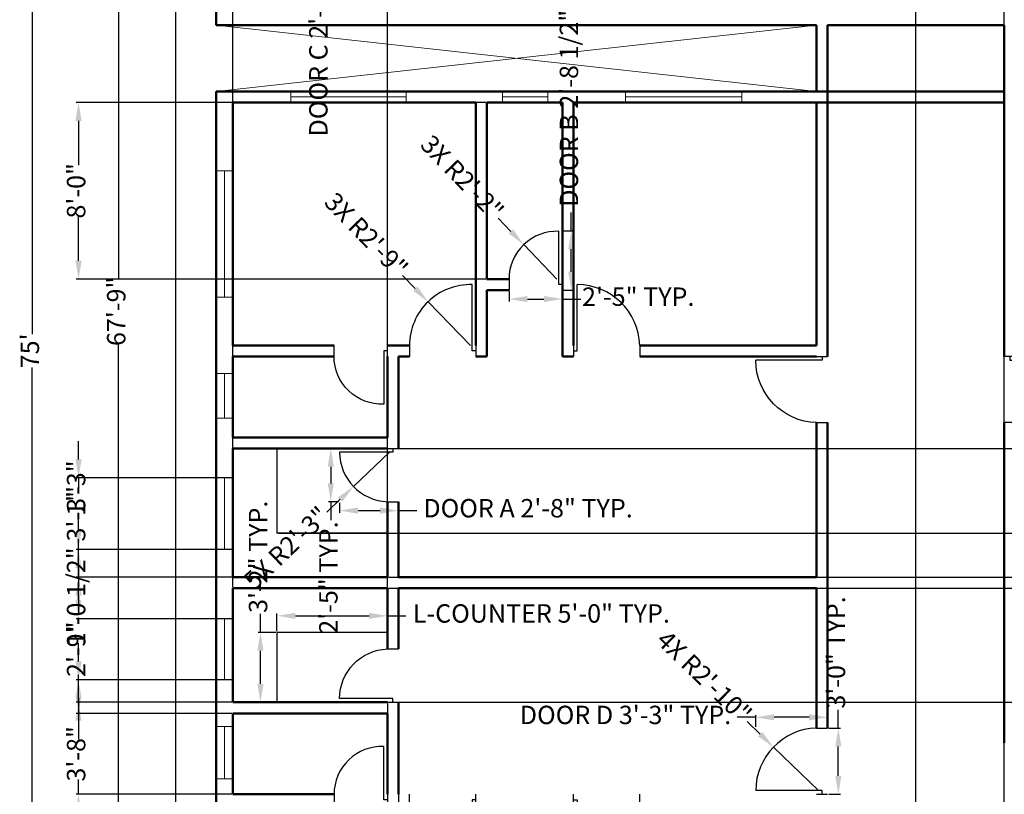
# Model space of a CAD drawing. Units: inches. Extents: x 3237 to 4201, y 2949 to 4053.
# Tile 2 of 5: x 3237 to 3772, y 3217 to 3638. Entities that reach past the tile are written whole.
import ezdxf

# ---------------------------------------------------------------- set-up
doc = ezdxf.new("R2010")
doc.units = ezdxf.units.IN
for name, color, linetype, lineweight in [('A-ANNO-DIMS', 2, 'Continuous', 18), ('A-DOOR', 3, 'Continuous', 25), ('A-FLOR-CASE', 8, 'Continuous', 25), ('A-FLOR-OPEN', 8, 'Continuous', 13), ('A-GLAZ', 4, 'Continuous', 18), ('A-WALL', 7, 'Continuous', 50), ('C-PROP', 6, 'Continuous', 25)]:
    doc.layers.add(name, color=color, linetype=linetype, lineweight=lineweight)
doc.styles.get("Standard").update_dxf_attribs({"font": 'arial.ttf'})
doc.dimstyles.new('ISO-25', dxfattribs={"dimtxt": 10, "dimasz": 10, "dimexe": 1.25, "dimexo": 0.625, "dimtad": 0, "dimdec": 0, "dimlunit": 3, "dimtxsty": 'Standard', "dimcen": 2.5, "dimadec": 0, "dimazin": 0, "dimtfac": 1, "dimtdec": 0, "dimtmove": 0, "dimatfit": 3, "dimfxl": 1, "dimarcsym": 0})

# ---------------------------------------------------------------- blocks, each defined once
blk = doc.blocks.new('*D2')
at = {"layer": 'A-ANNO-DIMS', "color": 0, "lineweight": -2, "transparency": 16777216}
for p, q in [((3320.9, 3907.98), (3242.34, 3907.98)), ((3243.59, 3897.98), (3243.59, 3467.05)), ((3243.59, 3017.98), (3243.59, 3448.91)), ((3320.9, 3007.98), (3242.34, 3007.98))]:
    blk.add_line(p, q, dxfattribs=at)
at = {"layer": 'A-ANNO-DIMS', "color": 0, "transparency": 16777216}
for points in [[(3241.92, 3897.98), (3245.26, 3897.98), (3243.59, 3907.98)], [(3241.92, 3017.98), (3245.26, 3017.98), (3243.59, 3007.98)]]:
    blk.add_solid(points, dxfattribs=at)
at = {"layer": 'Defpoints', "color": 0, "transparency": 16777216}
for p in [(3321.52, 3907.98), (3243.59, 3007.98), (3321.52, 3007.98)]:
    blk.add_point(p, dxfattribs=at)
at = {"layer": 'A-ANNO-DIMS', "color": 0, "transparency": 16777216, "insert": (3243.59, 3457.98), "char_height": 10, "attachment_point": 5, "rotation": 90}
blk.add_mtext("75'", dxfattribs=at)
blk = doc.blocks.new('*D4')
at = {"layer": 'A-ANNO-DIMS', "color": 0, "lineweight": -2, "transparency": 16777216}
for p, q in [((3342.9, 3885.98), (3289.25, 3885.98)), ((3290.5, 3875.98), (3290.5, 3497.31)), ((3290.5, 3082.98), (3290.5, 3461.65)), ((3342.9, 3072.98), (3289.25, 3072.98))]:
    blk.add_line(p, q, dxfattribs=at)
at = {"layer": 'A-ANNO-DIMS', "color": 0, "transparency": 16777216}
for points in [[(3288.84, 3875.98), (3292.17, 3875.98), (3290.5, 3885.98)], [(3288.84, 3082.98), (3292.17, 3082.98), (3290.5, 3072.98)]]:
    blk.add_solid(points, dxfattribs=at)
at = {"layer": 'Defpoints', "color": 0, "transparency": 16777216}
for p in [(3343.52, 3885.98), (3290.5, 3072.98), (3343.52, 3072.98)]:
    blk.add_point(p, dxfattribs=at)
at = {"layer": 'A-ANNO-DIMS', "color": 0, "transparency": 16777216, "insert": (3290.5, 3479.48), "char_height": 10, "attachment_point": 5, "rotation": 90}
blk.add_mtext('67\'-9"', dxfattribs=at)
blk = doc.blocks.new('DOOR-29-OFFSET-A')
for p, q in [((0, 26), (0, 32)), ((0, 29), (2, 29)), ((2, 29), (2, 0)), ((29, 26), (29, 32))]:
    blk.add_line(p, q)
blk.add_arc((2, 27.02), 27.02, 270, 357.8382)
blk = doc.blocks.new('DOOR-36-OFFSET-A')
for p, q in [((2, 3), (2, 39)), ((0, 6), (0, 0)), ((36, 6), (36, 0)), ((0, 3), (2, 3))]:
    blk.add_line(p, q)
blk.add_arc((2, 4.98), 34.02, 1.7102, 90)
blk = doc.blocks.new('DOOR-29-OFFSET-B')
for p, q in [((27, 3), (27, 32)), ((0, 6), (0, 0)), ((29, 6), (29, 0)), ((29, 3), (27, 3))]:
    blk.add_line(p, q)
blk.add_arc((26.02, 6), 26.02, 87.8382, 180)
blk = doc.blocks.new('DOOR-36-OFFSET-B')
for p, q in [((34, 3), (34, 39)), ((0, 6), (0, 0)), ((36, 6), (36, 0)), ((36, 3), (34, 3))]:
    blk.add_line(p, q)
blk.add_arc((33.01, 6), 33.01, 88.2898, 180)
blk = doc.blocks.new('WIN-68p61IN')
for p, q in [((0, 68.61), (9, 68.61)), ((4.5, 0), (4.5, 68.61)), ((0, 0), (9, 0))]:
    blk.add_line(p, q)
blk = doc.blocks.new('COUNTER-L-60x38')
for p, q in [((60, 38), (0, 38)), ((0, 38), (0, 0))]:
    blk.add_line(p, q)
blk = doc.blocks.new('*D15')
at = {"layer": 'A-ANNO-DIMS', "color": 0, "lineweight": -2, "transparency": 16777216}
for p, q in [((3410.52, 3375.35), (3410.52, 3369.93)), ((3442.52, 3375.35), (3442.52, 3369.93)), ((3420.52, 3371.18), (3432.52, 3371.18)), ((3442.52, 3371.18), (3452.52, 3371.18))]:
    blk.add_line(p, q, dxfattribs=at)
at = {"layer": 'A-ANNO-DIMS', "color": 0, "transparency": 16777216}
for points in [[(3420.52, 3372.85), (3420.52, 3369.51), (3410.52, 3371.18)], [(3432.52, 3372.85), (3432.52, 3369.51), (3442.52, 3371.18)]]:
    blk.add_solid(points, dxfattribs=at)
at = {"layer": 'Defpoints', "color": 0, "transparency": 16777216}
for p in [(3410.52, 3375.98), (3442.52, 3375.98), (3442.52, 3371.18)]:
    blk.add_point(p, dxfattribs=at)
at = {"layer": 'A-ANNO-DIMS', "color": 0, "transparency": 16777216, "insert": (3512.87, 3371.18), "char_height": 10, "attachment_point": 5}
blk.add_mtext('DOOR A 2\'-8" TYP.', dxfattribs=at)
blk = doc.blocks.new('*D16')
at = {"layer": 'A-ANNO-DIMS', "color": 0, "lineweight": -2, "transparency": 16777216}
for p, q in [((3409.9, 3404.98), (3404.47, 3404.98)), ((3405.72, 3394.98), (3405.72, 3385.98)), ((3409.9, 3375.98), (3404.47, 3375.98)), ((3405.72, 3375.98), (3405.72, 3365.98))]:
    blk.add_line(p, q, dxfattribs=at)
at = {"layer": 'A-ANNO-DIMS', "color": 0, "transparency": 16777216}
for points in [[(3404.06, 3394.98), (3407.39, 3394.98), (3405.72, 3404.98)], [(3404.06, 3385.98), (3407.39, 3385.98), (3405.72, 3375.98)]]:
    blk.add_solid(points, dxfattribs=at)
at = {"layer": 'Defpoints', "color": 0, "transparency": 16777216}
for p in [(3410.52, 3404.98), (3405.72, 3375.98), (3410.52, 3375.98)]:
    blk.add_point(p, dxfattribs=at)
at = {"layer": 'A-ANNO-DIMS', "color": 0, "transparency": 16777216, "insert": (3405.72, 3334.79), "char_height": 10, "attachment_point": 5, "rotation": 90}
blk.add_mtext('2\'-5" TYP.', dxfattribs=at)
blk = doc.blocks.new('*D17')
at = {"layer": 'A-ANNO-DIMS', "color": 0, "lineweight": -2, "transparency": 16777216}
for p, q in [((3536.36, 3523.25), (3536.36, 3533.25)), ((3532.15, 3523.25), (3537.61, 3523.25)), ((3536.36, 3500.98), (3536.36, 3513.25)), ((3532.15, 3490.98), (3537.61, 3490.98))]:
    blk.add_line(p, q, dxfattribs=at)
at = {"layer": 'A-ANNO-DIMS', "color": 0, "transparency": 16777216}
for points in [[(3534.7, 3513.25), (3538.03, 3513.25), (3536.36, 3523.25)], [(3534.7, 3500.98), (3538.03, 3500.98), (3536.36, 3490.98)]]:
    blk.add_solid(points, dxfattribs=at)
at = {"layer": 'Defpoints', "color": 0, "transparency": 16777216}
for p in [(3531.52, 3523.25), (3536.36, 3523.25), (3531.52, 3490.98)]:
    blk.add_point(p, dxfattribs=at)
at = {"layer": 'A-ANNO-DIMS', "color": 0, "transparency": 16777216, "insert": (3536.36, 3605.25), "char_height": 10, "attachment_point": 5, "rotation": 90}
blk.add_mtext('DOOR B 2\'-8 1/2" TYP.', dxfattribs=at)
blk = doc.blocks.new('*D18')
at = {"layer": 'A-ANNO-DIMS', "color": 0, "lineweight": -2, "transparency": 16777216}
for p, q in [((3502.52, 3490.35), (3502.52, 3484.89)), ((3531.52, 3490.35), (3531.52, 3484.89)), ((3512.52, 3486.14), (3521.52, 3486.14)), ((3531.52, 3486.14), (3541.52, 3486.14))]:
    blk.add_line(p, q, dxfattribs=at)
at = {"layer": 'A-ANNO-DIMS', "color": 0, "transparency": 16777216}
for points in [[(3512.52, 3487.81), (3512.52, 3484.47), (3502.52, 3486.14)], [(3521.52, 3487.81), (3521.52, 3484.47), (3531.52, 3486.14)]]:
    blk.add_solid(points, dxfattribs=at)
at = {"layer": 'Defpoints', "color": 0, "transparency": 16777216}
for p in [(3502.52, 3490.98), (3531.52, 3490.98), (3531.52, 3486.14)]:
    blk.add_point(p, dxfattribs=at)
at = {"layer": 'A-ANNO-DIMS', "color": 0, "transparency": 16777216, "insert": (3572.71, 3486.14), "char_height": 10, "attachment_point": 5}
blk.add_mtext('2\'-5" TYP.', dxfattribs=at)
blk = doc.blocks.new('*D19')
at = {"layer": 'A-ANNO-DIMS', "color": 0, "lineweight": -2, "transparency": 16777216}
for p, q in [((3404.9, 3744.98), (3399.02, 3744.98)), ((3400.27, 3734.98), (3400.27, 3719.98)), ((3404.9, 3709.98), (3399.02, 3709.98)), ((3400.27, 3709.98), (3400.27, 3699.98))]:
    blk.add_line(p, q, dxfattribs=at)
at = {"layer": 'A-ANNO-DIMS', "color": 0, "transparency": 16777216}
for points in [[(3398.61, 3734.98), (3401.94, 3734.98), (3400.27, 3744.98)], [(3398.61, 3719.98), (3401.94, 3719.98), (3400.27, 3709.98)]]:
    blk.add_solid(points, dxfattribs=at)
at = {"layer": 'Defpoints', "color": 0, "transparency": 16777216}
for p in [(3405.52, 3744.98), (3400.27, 3709.98), (3405.52, 3709.98)]:
    blk.add_point(p, dxfattribs=at)
at = {"layer": 'A-ANNO-DIMS', "color": 0, "transparency": 16777216, "insert": (3400.27, 3635.36), "char_height": 10, "attachment_point": 5, "rotation": 90}
blk.add_mtext('DOOR C 2\'-11" TYP.', dxfattribs=at)
blk = doc.blocks.new('*D21')
at = {"layer": 'A-ANNO-DIMS', "color": 0, "lineweight": -2, "transparency": 16777216}
for p, q in [((3636.52, 3258.83), (3626.52, 3258.83)), ((3636.52, 3253.6), (3636.52, 3260.08)), ((3665.52, 3258.83), (3646.52, 3258.83)), ((3675.52, 3253.6), (3675.52, 3260.08))]:
    blk.add_line(p, q, dxfattribs=at)
at = {"layer": 'A-ANNO-DIMS', "color": 0, "transparency": 16777216}
for points in [[(3646.52, 3260.5), (3646.52, 3257.16), (3636.52, 3258.83)], [(3665.52, 3260.5), (3665.52, 3257.16), (3675.52, 3258.83)]]:
    blk.add_solid(points, dxfattribs=at)
at = {"layer": 'Defpoints', "color": 0, "transparency": 16777216}
for p in [(3636.52, 3258.83), (3636.52, 3252.98), (3675.52, 3252.98)]:
    blk.add_point(p, dxfattribs=at)
at = {"layer": 'A-ANNO-DIMS', "color": 0, "transparency": 16777216, "insert": (3565.79, 3258.83), "char_height": 10, "attachment_point": 5}
blk.add_mtext('DOOR D 3\'-3" TYP.', dxfattribs=at)
blk = doc.blocks.new('*D22')
at = {"layer": 'A-ANNO-DIMS', "color": 0, "lineweight": -2, "transparency": 16777216}
for p, q in [((3681.37, 3252.98), (3681.37, 3262.98)), ((3676.15, 3252.98), (3682.62, 3252.98)), ((3681.37, 3226.98), (3681.37, 3242.98)), ((3676.15, 3216.98), (3682.62, 3216.98))]:
    blk.add_line(p, q, dxfattribs=at)
at = {"layer": 'A-ANNO-DIMS', "color": 0, "transparency": 16777216}
for points in [[(3679.71, 3242.98), (3683.04, 3242.98), (3681.37, 3252.98)], [(3679.71, 3226.98), (3683.04, 3226.98), (3681.37, 3216.98)]]:
    blk.add_solid(points, dxfattribs=at)
at = {"layer": 'Defpoints', "color": 0, "transparency": 16777216}
for p in [(3675.52, 3252.98), (3681.37, 3252.98), (3675.52, 3216.98)]:
    blk.add_point(p, dxfattribs=at)
at = {"layer": 'A-ANNO-DIMS', "color": 0, "transparency": 16777216, "insert": (3681.37, 3294.08), "char_height": 10, "attachment_point": 5, "rotation": 90}
blk.add_mtext('3\'-0" TYP.', dxfattribs=at)
blk = doc.blocks.new('*D33')
at = {"layer": 'A-ANNO-DIMS', "color": 0, "lineweight": -2, "transparency": 16777216}
for p, q in [((3376.52, 3305.6), (3376.52, 3315.23)), ((3386.52, 3313.98), (3426.52, 3313.98)), ((3436.52, 3305.6), (3436.52, 3315.23)), ((3436.52, 3313.98), (3446.52, 3313.98))]:
    blk.add_line(p, q, dxfattribs=at)
at = {"layer": 'A-ANNO-DIMS', "color": 0, "transparency": 16777216}
for points in [[(3386.52, 3315.65), (3386.52, 3312.31), (3376.52, 3313.98)], [(3426.52, 3315.65), (3426.52, 3312.31), (3436.52, 3313.98)]]:
    blk.add_solid(points, dxfattribs=at)
at = {"layer": 'Defpoints', "color": 0, "transparency": 16777216}
for p in [(3436.52, 3313.98), (3376.52, 3304.98), (3436.52, 3304.98)]:
    blk.add_point(p, dxfattribs=at)
at = {"layer": 'A-ANNO-DIMS', "color": 0, "transparency": 16777216, "insert": (3520.09, 3313.98), "char_height": 10, "attachment_point": 5}
blk.add_mtext('L-COUNTER 5\'-0" TYP.', dxfattribs=at)
blk = doc.blocks.new('*D34')
at = {"layer": 'A-ANNO-DIMS', "color": 0, "lineweight": -2, "transparency": 16777216}
for p, q in [((3367.52, 3304.98), (3367.52, 3314.98)), ((3375.9, 3304.98), (3366.27, 3304.98)), ((3367.52, 3276.98), (3367.52, 3294.98)), ((3375.9, 3266.98), (3366.27, 3266.98))]:
    blk.add_line(p, q, dxfattribs=at)
at = {"layer": 'A-ANNO-DIMS', "color": 0, "transparency": 16777216}
for points in [[(3365.86, 3294.98), (3369.19, 3294.98), (3367.52, 3304.98)], [(3365.86, 3276.98), (3369.19, 3276.98), (3367.52, 3266.98)]]:
    blk.add_solid(points, dxfattribs=at)
at = {"layer": 'Defpoints', "color": 0, "transparency": 16777216}
for p in [(3367.52, 3304.98), (3376.52, 3304.98), (3376.52, 3266.98)]:
    blk.add_point(p, dxfattribs=at)
at = {"layer": 'A-ANNO-DIMS', "color": 0, "transparency": 16777216, "insert": (3367.52, 3346.08), "char_height": 10, "attachment_point": 5, "rotation": 90}
blk.add_mtext('3\'-2" TYP.', dxfattribs=at)
blk = doc.blocks.new('*D60')
at = {"layer": 'A-ANNO-DIMS', "color": 0, "lineweight": -2, "transparency": 16777216}
for p, q in [((3268.72, 3270.98), (3268.72, 3280.98)), ((3351.9, 3260.98), (3267.47, 3260.98)), ((3268.72, 3260.98), (3268.72, 3252.89)), ((3268.72, 3216.98), (3268.72, 3225.07)), ((3351.9, 3216.98), (3267.47, 3216.98)), ((3268.72, 3206.98), (3268.72, 3196.98))]:
    blk.add_line(p, q, dxfattribs=at)
at = {"layer": 'A-ANNO-DIMS', "color": 0, "transparency": 16777216}
for points in [[(3267.06, 3270.98), (3270.39, 3270.98), (3268.72, 3260.98)], [(3267.06, 3206.98), (3270.39, 3206.98), (3268.72, 3216.98)]]:
    blk.add_solid(points, dxfattribs=at)
at = {"layer": 'Defpoints', "color": 0, "transparency": 16777216}
for p in [(3268.72, 3260.98), (3352.52, 3260.98), (3352.52, 3216.98)]:
    blk.add_point(p, dxfattribs=at)
at = {"layer": 'A-ANNO-DIMS', "color": 0, "transparency": 16777216, "insert": (3268.72, 3238.98), "char_height": 10, "attachment_point": 5, "rotation": 90}
blk.add_mtext('3\'-8"', dxfattribs=at)
blk = doc.blocks.new('*D61')
at = {"layer": 'A-ANNO-DIMS', "color": 0, "lineweight": -2, "transparency": 16777216}
for p, q in [((3437.15, 3328.98), (4187.57, 3328.98)), ((4186.32, 3318.98), (4186.32, 3311.9)), ((4186.32, 3276.98), (4186.32, 3284.06)), ((3437.15, 3266.98), (4187.57, 3266.98))]:
    blk.add_line(p, q, dxfattribs=at)
at = {"layer": 'A-ANNO-DIMS', "color": 0, "transparency": 16777216}
for points in [[(4184.66, 3318.98), (4187.99, 3318.98), (4186.32, 3328.98)], [(4184.66, 3276.98), (4187.99, 3276.98), (4186.32, 3266.98)]]:
    blk.add_solid(points, dxfattribs=at)
at = {"layer": 'Defpoints', "color": 0, "transparency": 16777216}
for p in [(3436.52, 3328.98), (4186.32, 3328.98), (3436.52, 3266.98)]:
    blk.add_point(p, dxfattribs=at)
at = {"layer": 'A-ANNO-DIMS', "color": 0, "transparency": 16777216, "insert": (4186.32, 3297.98), "char_height": 10, "attachment_point": 5, "rotation": 90}
blk.add_mtext('5\'-2"', dxfattribs=at)
blk = doc.blocks.new('*D62')
at = {"layer": 'A-ANNO-DIMS', "color": 0, "lineweight": -2, "transparency": 16777216}
for p, q in [((3437.15, 3404.98), (4187.57, 3404.98)), ((4186.32, 3394.98), (4186.32, 3387.78)), ((4186.32, 3344.98), (4186.32, 3352.18)), ((3437.15, 3334.98), (4187.57, 3334.98))]:
    blk.add_line(p, q, dxfattribs=at)
at = {"layer": 'A-ANNO-DIMS', "color": 0, "transparency": 16777216}
for points in [[(4184.66, 3394.98), (4187.99, 3394.98), (4186.32, 3404.98)], [(4184.66, 3344.98), (4187.99, 3344.98), (4186.32, 3334.98)]]:
    blk.add_solid(points, dxfattribs=at)
at = {"layer": 'Defpoints', "color": 0, "transparency": 16777216}
for p in [(3436.52, 3404.98), (4186.32, 3404.98), (3436.52, 3334.98)]:
    blk.add_point(p, dxfattribs=at)
at = {"layer": 'A-ANNO-DIMS', "color": 0, "transparency": 16777216, "insert": (4186.32, 3369.98), "char_height": 10, "attachment_point": 5, "rotation": 90}
blk.add_mtext('5\'-10"', dxfattribs=at)
blk = doc.blocks.new('*D72')
at = {"layer": 'A-ANNO-DIMS', "color": 0, "lineweight": -2, "transparency": 16777216}
for p, q in [((3489.9, 3592.98), (3267.47, 3592.98)), ((3268.72, 3582.98), (3268.72, 3558.9)), ((3268.72, 3506.98), (3268.72, 3531.06)), ((3489.9, 3496.98), (3267.47, 3496.98))]:
    blk.add_line(p, q, dxfattribs=at)
at = {"layer": 'A-ANNO-DIMS', "color": 0, "transparency": 16777216}
for points in [[(3267.06, 3582.98), (3270.39, 3582.98), (3268.72, 3592.98)], [(3267.06, 3506.98), (3270.39, 3506.98), (3268.72, 3496.98)]]:
    blk.add_solid(points, dxfattribs=at)
at = {"layer": 'Defpoints', "color": 0, "transparency": 16777216}
for p in [(3268.72, 3592.98), (3490.52, 3592.98), (3490.52, 3496.98)]:
    blk.add_point(p, dxfattribs=at)
at = {"layer": 'A-ANNO-DIMS', "color": 0, "transparency": 16777216, "insert": (3268.72, 3544.98), "char_height": 10, "attachment_point": 5, "rotation": 90}
blk.add_mtext('8\'-0"', dxfattribs=at)
blk = doc.blocks.new('*D73')
at = {"layer": 'A-ANNO-DIMS', "color": 0, "lineweight": -2, "transparency": 16777216}
for p, q in [((3352.52, 3329.6), (3352.52, 3962.03)), ((3362.52, 3960.78), (3380.65, 3960.78)), ((3426.52, 3960.78), (3408.4, 3960.78)), ((3436.52, 3329.6), (3436.52, 3962.03))]:
    blk.add_line(p, q, dxfattribs=at)
at = {"layer": 'A-ANNO-DIMS', "color": 0, "transparency": 16777216}
for points in [[(3362.52, 3962.45), (3362.52, 3959.11), (3352.52, 3960.78)], [(3426.52, 3962.45), (3426.52, 3959.11), (3436.52, 3960.78)]]:
    blk.add_solid(points, dxfattribs=at)
at = {"layer": 'Defpoints', "color": 0, "transparency": 16777216}
for p in [(3436.52, 3960.78), (3352.52, 3328.98), (3436.52, 3328.98)]:
    blk.add_point(p, dxfattribs=at)
at = {"layer": 'A-ANNO-DIMS', "color": 0, "transparency": 16777216, "insert": (3394.52, 3960.78), "char_height": 10, "attachment_point": 5}
blk.add_mtext('7\'-0"', dxfattribs=at)
blk = doc.blocks.new('*D74')
at = {"layer": 'A-ANNO-DIMS', "color": 0, "lineweight": -2, "transparency": 16777216}
for p, q in [((4186.32, 3414.98), (4186.32, 3424.98)), ((3377.15, 3404.98), (4187.57, 3404.98)), ((4186.32, 3404.98), (4186.32, 3399.78)), ((4186.32, 3358.98), (4186.32, 3364.18)), ((3377.15, 3358.98), (4187.57, 3358.98)), ((4186.32, 3348.98), (4186.32, 3338.98))]:
    blk.add_line(p, q, dxfattribs=at)
at = {"layer": 'A-ANNO-DIMS', "color": 0, "transparency": 16777216}
for points in [[(4184.66, 3414.98), (4187.99, 3414.98), (4186.32, 3404.98)], [(4184.66, 3348.98), (4187.99, 3348.98), (4186.32, 3358.98)]]:
    blk.add_solid(points, dxfattribs=at)
at = {"layer": 'Defpoints', "color": 0, "transparency": 16777216}
for p in [(3376.52, 3404.98), (4186.32, 3404.98), (3376.52, 3358.98)]:
    blk.add_point(p, dxfattribs=at)
at = {"layer": 'A-ANNO-DIMS', "color": 0, "transparency": 16777216, "insert": (4186.32, 3381.98), "char_height": 10, "attachment_point": 5, "rotation": 90}
blk.add_mtext('3\'-10"', dxfattribs=at)
blk = doc.blocks.new('*D75')
at = {"layer": 'A-ANNO-DIMS', "color": 0, "lineweight": -2, "transparency": 16777216}
for p, q in [((3436.52, 3266.35), (3436.52, 2953.93)), ((3442.52, 3266.35), (3442.52, 2953.93)), ((3426.52, 2955.18), (3416.52, 2955.18)), ((3436.52, 2955.18), (3442.52, 2955.18)), ((3452.52, 2955.18), (3462.52, 2955.18))]:
    blk.add_line(p, q, dxfattribs=at)
at = {"layer": 'A-ANNO-DIMS', "color": 0, "transparency": 16777216}
for points in [[(3426.52, 2956.85), (3426.52, 2953.51), (3436.52, 2955.18)], [(3452.52, 2956.85), (3452.52, 2953.51), (3442.52, 2955.18)]]:
    blk.add_solid(points, dxfattribs=at)
at = {"layer": 'Defpoints', "color": 0, "transparency": 16777216}
for p in [(3436.52, 3266.98), (3442.52, 3266.98), (3442.52, 2955.18)]:
    blk.add_point(p, dxfattribs=at)
at = {"layer": 'A-ANNO-DIMS', "color": 0, "transparency": 16777216, "insert": (3476.44, 2955.18), "char_height": 10, "attachment_point": 5}
blk.add_mtext('0\'-6"', dxfattribs=at)
blk = doc.blocks.new('*D76')
at = {"layer": 'A-ANNO-DIMS', "color": 0, "lineweight": -2, "transparency": 16777216}
for p, q in [((3268.72, 3322.42), (3268.72, 3332.42)), ((3351.9, 3312.42), (3267.47, 3312.42)), ((3268.72, 3312.42), (3268.72, 3309.84)), ((3351.9, 3279.25), (3267.47, 3279.25)), ((3268.72, 3279.25), (3268.72, 3281.83)), ((3268.72, 3269.25), (3268.72, 3259.25))]:
    blk.add_line(p, q, dxfattribs=at)
at = {"layer": 'A-ANNO-DIMS', "color": 0, "transparency": 16777216}
for points in [[(3267.06, 3322.42), (3270.39, 3322.42), (3268.72, 3312.42)], [(3267.06, 3269.25), (3270.39, 3269.25), (3268.72, 3279.25)]]:
    blk.add_solid(points, dxfattribs=at)
at = {"layer": 'Defpoints', "color": 0, "transparency": 16777216}
for p in [(3268.72, 3312.42), (3352.52, 3312.42), (3352.52, 3279.25)]:
    blk.add_point(p, dxfattribs=at)
at = {"layer": 'A-ANNO-DIMS', "color": 0, "transparency": 16777216, "insert": (3268.72, 3295.84), "char_height": 10, "attachment_point": 5, "rotation": 90}
blk.add_mtext('2\'-9"', dxfattribs=at)
blk = doc.blocks.new('*D77')
at = {"layer": 'A-ANNO-DIMS', "color": 0, "lineweight": -2, "transparency": 16777216}
for p, q in [((3268.72, 3289.25), (3268.72, 3299.25)), ((3351.9, 3279.25), (3267.47, 3279.25)), ((3268.72, 3266.98), (3268.72, 3279.25)), ((3351.9, 3266.98), (3267.47, 3266.98)), ((3268.72, 3256.98), (3268.72, 3246.98))]:
    blk.add_line(p, q, dxfattribs=at)
at = {"layer": 'A-ANNO-DIMS', "color": 0, "transparency": 16777216}
for points in [[(3267.06, 3289.25), (3270.39, 3289.25), (3268.72, 3279.25)], [(3267.06, 3256.98), (3270.39, 3256.98), (3268.72, 3266.98)]]:
    blk.add_solid(points, dxfattribs=at)
at = {"layer": 'Defpoints', "color": 0, "transparency": 16777216}
for p in [(3268.72, 3279.25), (3352.52, 3279.25), (3352.52, 3266.98)]:
    blk.add_point(p, dxfattribs=at)
at = {"layer": 'A-ANNO-DIMS', "color": 0, "transparency": 16777216, "insert": (3268.72, 3324.35), "char_height": 10, "attachment_point": 5, "rotation": 90}
blk.add_mtext('1\'-0 1/2"', dxfattribs=at)
blk = doc.blocks.new('*D78')
at = {"layer": 'A-ANNO-DIMS', "color": 0, "lineweight": -2, "transparency": 16777216}
for p, q in [((3268.72, 3398.99), (3268.72, 3408.99)), ((3351.9, 3388.99), (3267.47, 3388.99)), ((3268.72, 3388.99), (3268.72, 3383.38)), ((3268.72, 3349.95), (3268.72, 3355.56)), ((3351.9, 3349.95), (3267.47, 3349.95)), ((3268.72, 3339.95), (3268.72, 3329.95))]:
    blk.add_line(p, q, dxfattribs=at)
at = {"layer": 'A-ANNO-DIMS', "color": 0, "transparency": 16777216}
for points in [[(3267.06, 3398.99), (3270.39, 3398.99), (3268.72, 3388.99)], [(3267.06, 3339.95), (3270.39, 3339.95), (3268.72, 3349.95)]]:
    blk.add_solid(points, dxfattribs=at)
at = {"layer": 'Defpoints', "color": 0, "transparency": 16777216}
for p in [(3268.72, 3388.99), (3352.52, 3388.99), (3352.52, 3349.95)]:
    blk.add_point(p, dxfattribs=at)
at = {"layer": 'A-ANNO-DIMS', "color": 0, "transparency": 16777216, "insert": (3268.72, 3369.47), "char_height": 10, "attachment_point": 5, "rotation": 90}
blk.add_mtext('3\'-3"', dxfattribs=at)
blk = doc.blocks.new('*D79')
at = {"layer": 'A-ANNO-DIMS', "color": 0, "lineweight": -2, "transparency": 16777216}
for p, q in [((3268.72, 3359.95), (3268.72, 3369.95)), ((3351.9, 3349.95), (3267.47, 3349.95)), ((3268.72, 3334.98), (3268.72, 3349.95)), ((3351.9, 3334.98), (3267.47, 3334.98)), ((3268.72, 3324.98), (3268.72, 3314.98))]:
    blk.add_line(p, q, dxfattribs=at)
at = {"layer": 'A-ANNO-DIMS', "color": 0, "transparency": 16777216}
for points in [[(3267.06, 3359.95), (3270.39, 3359.95), (3268.72, 3349.95)], [(3267.06, 3324.98), (3270.39, 3324.98), (3268.72, 3334.98)]]:
    blk.add_solid(points, dxfattribs=at)
at = {"layer": 'Defpoints', "color": 0, "transparency": 16777216}
for p in [(3268.72, 3349.95), (3352.52, 3349.95), (3352.52, 3334.98)]:
    blk.add_point(p, dxfattribs=at)
at = {"layer": 'A-ANNO-DIMS', "color": 0, "transparency": 16777216, "insert": (3268.72, 3383.39), "char_height": 10, "attachment_point": 5, "rotation": 90}
blk.add_mtext('1\'-3"', dxfattribs=at)
blk = doc.blocks.new('*D83')
at = {"layer": 'A-ANNO-DIMS', "color": 0, "lineweight": -2, "transparency": 16777216}
for p, q in [((3713.52, 3960.78), (3703.52, 3960.78)), ((3723.52, 3193.4), (3723.52, 3962.03)), ((3723.52, 3960.78), (3733.4, 3960.78)), ((3771.52, 3960.78), (3761.64, 3960.78)), ((3771.52, 3193.4), (3771.52, 3962.03)), ((3781.52, 3960.78), (3791.52, 3960.78))]:
    blk.add_line(p, q, dxfattribs=at)
at = {"layer": 'A-ANNO-DIMS', "color": 0, "transparency": 16777216}
for points in [[(3713.52, 3962.45), (3713.52, 3959.11), (3723.52, 3960.78)], [(3781.52, 3962.45), (3781.52, 3959.11), (3771.52, 3960.78)]]:
    blk.add_solid(points, dxfattribs=at)
at = {"layer": 'Defpoints', "color": 0, "transparency": 16777216}
for p in [(3771.52, 3960.78), (3723.52, 3192.78), (3771.52, 3192.78)]:
    blk.add_point(p, dxfattribs=at)
at = {"layer": 'A-ANNO-DIMS', "color": 0, "transparency": 16777216, "insert": (3747.52, 3960.78), "char_height": 10, "attachment_point": 5}
blk.add_mtext('4\'-0"', dxfattribs=at)
blk = doc.blocks.new('*D88')
at = {"layer": 'A-ANNO-DIMS', "color": 0, "lineweight": -2, "transparency": 16777216}
for p, q in [((3444.61, 3499.02), (3451.58, 3491.85)), ((3481.54, 3460.98), (3458.54, 3484.67))]:
    blk.add_line(p, q, dxfattribs=at)
at = {"layer": 'A-ANNO-DIMS', "color": 0, "transparency": 16777216}
blk.add_solid([(3452.77, 3493.01), (3450.38, 3490.69), (3458.54, 3484.67)], dxfattribs=at)
at = {"layer": 'Defpoints', "color": 0, "transparency": 16777216}
for p in [(3458.54, 3484.67), (3481.54, 3460.98)]:
    blk.add_point(p, dxfattribs=at)
at = {"layer": 'A-ANNO-DIMS', "color": 0, "transparency": 16777216, "insert": (3424.11, 3520.15), "char_height": 10, "attachment_point": 5, "rotation": 314.1447}
blk.add_mtext('3X R2\'-9"', dxfattribs=at)
blk = doc.blocks.new('*D89')
at = {"layer": 'A-ANNO-DIMS', "color": 0, "lineweight": -2, "transparency": 16777216}
for p, q in [((3631.78, 3256.6), (3638.95, 3249.63)), ((3670.54, 3218.98), (3646.13, 3242.67))]:
    blk.add_line(p, q, dxfattribs=at)
at = {"layer": 'A-ANNO-DIMS', "color": 0, "transparency": 16777216}
blk.add_solid([(3640.11, 3250.83), (3637.79, 3248.44), (3646.13, 3242.67)], dxfattribs=at)
at = {"layer": 'Defpoints', "color": 0, "transparency": 16777216}
for p in [(3646.13, 3242.67), (3670.54, 3218.98)]:
    blk.add_point(p, dxfattribs=at)
at = {"layer": 'A-ANNO-DIMS', "color": 0, "transparency": 16777216, "insert": (3607.71, 3279.95), "char_height": 10, "attachment_point": 5, "rotation": 315.8558}
blk.add_mtext('4X R2\'-10"', dxfattribs=at)
blk = doc.blocks.new('*D90')
at = {"layer": 'A-ANNO-DIMS', "color": 0, "lineweight": -2, "transparency": 16777216}
for p, q in [((3437.54, 3402.98), (3418.08, 3384.24)), ((3403.67, 3370.37), (3410.87, 3377.3))]:
    blk.add_line(p, q, dxfattribs=at)
at = {"layer": 'A-ANNO-DIMS', "color": 0, "transparency": 16777216}
blk.add_solid([(3409.72, 3378.5), (3412.03, 3376.1), (3418.08, 3384.24)], dxfattribs=at)
at = {"layer": 'Defpoints', "color": 0, "transparency": 16777216}
for p in [(3437.54, 3402.98), (3418.08, 3384.24)]:
    blk.add_point(p, dxfattribs=at)
at = {"layer": 'A-ANNO-DIMS', "color": 0, "transparency": 16777216, "insert": (3382.46, 3349.94), "char_height": 10, "attachment_point": 5, "rotation": 43.9183}
blk.add_mtext('5X R2\'-3"', dxfattribs=at)
blk = doc.blocks.new('*D91')
at = {"layer": 'A-ANNO-DIMS', "color": 0, "lineweight": -2, "transparency": 16777216}
for p, q in [((3496.62, 3530.13), (3503.56, 3522.92)), ((3528.54, 3496.98), (3510.49, 3515.72))]:
    blk.add_line(p, q, dxfattribs=at)
at = {"layer": 'A-ANNO-DIMS', "color": 0, "transparency": 16777216}
blk.add_solid([(3504.76, 3524.08), (3502.36, 3521.77), (3510.49, 3515.72)], dxfattribs=at)
at = {"layer": 'Defpoints', "color": 0, "transparency": 16777216}
for p in [(3510.49, 3515.72), (3528.54, 3496.98)]:
    blk.add_point(p, dxfattribs=at)
at = {"layer": 'A-ANNO-DIMS', "color": 0, "transparency": 16777216, "insert": (3476.2, 3551.34), "char_height": 10, "attachment_point": 5, "rotation": 313.919}
blk.add_mtext('3X R2\'-2"', dxfattribs=at)

msp = doc.modelspace()

# ---------------------------------------------------------------- linework, layer by layer
at = {"layer": 'A-FLOR-CASE'}
for p in [(3376.52, 3404.98), (3436.52, 3358.98)]:
    msp.add_line(p, (3376.52, 3358.98), dxfattribs=at)
at = {"layer": 'A-FLOR-OPEN'}
for p, q in [((3343.52, 3598.98), (3669.52, 3634.98)), ((3669.52, 3598.98), (3343.52, 3634.98))]:
    msp.add_line(p, q, dxfattribs=at)
at = {"layer": 'A-GLAZ'}
for p, q in [((3384.01, 3598.98), (3384.01, 3592.98)), ((3446.62, 3592.98), (3446.62, 3598.98)), ((3446.62, 3598.98), (3446.62, 3595.98)), ((3499.03, 3592.98), (3499.03, 3598.98)), ((3523.52, 3592.98), (3523.52, 3598.98)), ((3565.81, 3592.98), (3565.81, 3598.98)), ((3628.89, 3592.98), (3628.89, 3598.98)), ((3446.62, 3595.98), (3384.01, 3595.98)), ((3523.52, 3595.98), (3499.03, 3595.98)), ((3628.89, 3595.98), (3565.81, 3595.98)), ((3384.01, 3592.98), (3446.62, 3592.98)), ((3343.52, 3487.24), (3343.52, 3555.85)), ((3352.52, 3555.85), (3348.02, 3555.85)), ((3352.52, 3445.7), (3343.52, 3445.7)), ((3348.02, 3445.7), (3348.02, 3421.34)), ((3352.52, 3421.34), (3343.52, 3421.34)), ((3352.52, 3388.99), (3343.52, 3388.99)), ((3348.02, 3388.99), (3348.02, 3349.95)), ((3352.52, 3349.95), (3343.52, 3349.95)), ((3352.52, 3312.42), (3343.52, 3312.42)), ((3348.02, 3312.42), (3348.02, 3279.25)), ((3352.52, 3279.25), (3343.52, 3279.25)), ((3352.52, 3253.75), (3343.52, 3253.75)), ((3348.02, 3253.75), (3348.02, 3225.31)), ((3352.52, 3225.31), (3343.52, 3225.31))]:
    msp.add_line(p, q, dxfattribs=at)
at = {"layer": 'A-WALL'}
for p, q in [((3343.52, 3885.98), (3343.52, 3634.98)), ((3352.52, 3634.98), (3343.52, 3634.98)), ((3669.52, 3634.98), (3352.52, 3634.98)), ((3669.52, 3634.98), (3669.52, 3598.98)), ((3669.52, 3634.98), (3669.52, 3598.98)), ((3675.52, 3634.98), (3675.52, 3454.98)), ((3771.52, 3634.98), (3675.52, 3634.98)), ((3771.52, 3634.98), (3771.52, 3454.98)), ((3352.52, 3598.98), (3343.52, 3598.98)), ((3343.52, 3598.98), (3343.52, 3072.98)), ((3771.52, 3598.98), (3352.52, 3598.98)), ((3352.52, 3592.98), (3352.52, 3460.98)), ((3484.52, 3592.98), (3352.52, 3592.98)), ((3484.52, 3592.98), (3484.52, 3460.98)), ((3484.52, 3592.98), (3484.52, 3460.98)), ((3490.52, 3592.98), (3490.52, 3496.98)), ((3531.52, 3592.98), (3490.52, 3592.98)), ((3531.52, 3592.98), (3531.52, 3460.98)), ((3537.52, 3592.98), (3537.52, 3460.98)), ((3771.52, 3592.98), (3537.52, 3592.98)), ((3669.52, 3592.98), (3669.52, 3460.98)), ((3502.52, 3496.98), (3490.52, 3496.98)), ((3502.52, 3490.98), (3490.52, 3490.98)), ((3490.52, 3490.98), (3490.52, 3460.98)), ((3407.52, 3460.98), (3352.52, 3460.98)), ((3448.52, 3460.98), (3436.52, 3460.98)), ((3490.52, 3460.98), (3490.52, 3454.98)), ((3531.52, 3460.98), (3531.52, 3454.98)), ((3669.52, 3460.98), (3573.52, 3460.98)), ((3352.52, 3454.98), (3352.52, 3410.98)), ((3407.52, 3454.98), (3352.52, 3454.98)), ((3436.52, 3454.98), (3436.52, 3410.98)), ((3442.52, 3454.98), (3442.52, 3404.98)), ((3448.52, 3454.98), (3442.52, 3454.98)), ((3490.52, 3454.98), (3484.52, 3454.98)), ((3537.52, 3454.98), (3531.52, 3454.98)), ((3669.52, 3454.98), (3573.52, 3454.98)), ((3669.52, 3418.98), (3669.52, 3334.98)), ((3675.52, 3418.98), (3675.52, 3252.98)), ((3771.52, 3418.98), (3771.52, 3244.98)), ((3436.52, 3410.98), (3352.52, 3410.98)), ((3436.52, 3404.98), (3352.52, 3404.98)), ((3352.52, 3404.98), (3352.52, 3334.98)), ((3436.52, 3375.98), (3436.52, 3334.98)), ((3442.52, 3375.98), (3442.52, 3334.98)), ((3436.52, 3334.98), (3352.52, 3334.98)), ((3484.52, 3334.98), (3442.52, 3334.98)), ((3484.52, 3334.98), (3492.31, 3334.98)), ((3669.52, 3334.98), (3490.52, 3334.98)), ((3352.52, 3328.98), (3352.52, 3266.98)), ((3436.52, 3328.98), (3352.52, 3328.98)), ((3436.52, 3328.98), (3436.52, 3295.98)), ((3669.52, 3328.98), (3442.52, 3328.98)), ((3442.52, 3328.98), (3442.52, 3295.98)), ((3669.52, 3328.98), (3669.52, 3252.98)), ((3436.52, 3266.98), (3352.52, 3266.98)), ((3442.52, 3266.98), (3442.52, 3216.98)), ((3436.52, 3260.98), (3352.52, 3260.98)), ((3352.52, 3260.98), (3352.52, 3216.98)), ((3436.52, 3260.98), (3436.52, 3216.98)), ((3407.52, 3216.98), (3352.52, 3216.98))]:
    msp.add_line(p, q, dxfattribs=at)
at = {"layer": 'C-PROP'}
msp.add_line((3321.52, 3007.98), (3321.52, 3907.98), dxfattribs=at)

# ---------------------------------------------------------------- block references
at = {"layer": 'A-DOOR'}
for name, p in [('DOOR-29-OFFSET-B', (3502.52, 3490.98)), ('DOOR-36-OFFSET-B', (3448.52, 3454.98)), ('DOOR-36-OFFSET-A', (3537.52, 3454.98)), ('DOOR-29-OFFSET-B', (3407.52, 3210.98))]:
    msp.add_blockref(name, p, dxfattribs=at)
at = {"layer": 'A-DOOR', "extrusion": (0, 0, -1), "zscale": -1}
for name, p, rotation in [('DOOR-29-OFFSET-B', (-3407.52, 3460.98), 180), ('DOOR-36-OFFSET-A', (-3675.52, 3454.98), 269.9999999999968), ('DOOR-29-OFFSET-A', (-3410.52, 3266.98), 90.00000000000234), ('DOOR-36-OFFSET-B', (-3448.52, 3216.98), 180), ('DOOR-36-OFFSET-A', (-3537.52, 3216.98), 180)]:
    msp.add_blockref(name, p, dxfattribs=dict(at, rotation=rotation))
at = {"layer": 'A-DOOR'}
for name, p, rotation in [('DOOR-36-OFFSET-A', (3771.52, 3454.98), 270.0000000000005), ('DOOR-29-OFFSET-A', (3410.52, 3404.98), 270.0000000000013), ('DOOR-36-OFFSET-A', (3675.52, 3216.98), 89.99999999999756)]:
    msp.add_blockref(name, p, dxfattribs=dict(at, rotation=rotation))
at = {"layer": 'A-FLOR-CASE'}
msp.add_blockref('COUNTER-L-60x38', (3376.52, 3266.98), dxfattribs=at)
at = {"layer": 'A-GLAZ', "rotation": 180}
msp.add_blockref('WIN-68p61IN', (3352.52, 3555.85), dxfattribs=at)

# ---------------------------------------------------------------- dimensions: what is measured, and where the dimension line sits
at = {"layer": 'A-ANNO-DIMS'}
for base, p1, p2, picture, middle in [((3436.52, 3960.78), (3352.52, 3328.98), (3436.52, 3328.98), '*D73', (3394.52, 3960.78)), ((3771.52, 3960.78), (3723.52, 3192.78), (3771.52, 3192.78), '*D83', (3747.52, 3960.78)), ((3442.52, 2955.18), (3436.52, 3266.98), (3442.52, 3266.98), '*D75', (3476.44, 2955.18))]:
    dim = msp.add_linear_dim(base=base, p1=p1, p2=p2, dimstyle='ISO-25', override={"dimdec": 1, "dimlfac": 1, "dimrnd": 0, "dimzin": 1, "dimdsep": 46, "dimlunit": 4, "dimfrac": 2}, dxfattribs=at)
    dim.commit()
    dim.dimension.update_dxf_attribs({"geometry": picture, "text_midpoint": middle})
for base, p1, p2, override, picture, middle in [((3243.59, 3007.98), (3321.52, 3907.98), (3321.52, 3007.98), {"dimclrd": 0, "dimclre": 0, "dimclrt": 0}, '*D2', (3243.59, 3457.98)), ((3290.5, 3072.98), (3343.52, 3885.98), (3343.52, 3072.98), {"dimclrd": 0, "dimclre": 0, "dimclrt": 0}, '*D4', (3290.5, 3479.48)), ((3268.72, 3592.98), (3490.52, 3496.98), (3490.52, 3592.98), {"dimdec": 1, "dimlfac": 1, "dimrnd": 0, "dimzin": 1, "dimdsep": 46, "dimlunit": 4, "dimfrac": 2}, '*D72', (3268.72, 3544.98)), ((4186.32, 3404.98), (3376.52, 3358.98), (3376.52, 3404.98), {"dimdec": 1, "dimlfac": 1, "dimrnd": 0, "dimzin": 1, "dimdsep": 46, "dimlunit": 4, "dimfrac": 2}, '*D74', (4186.32, 3381.98)), ((3268.72, 3388.99), (3352.52, 3349.95), (3352.52, 3388.99), {"dimdec": 1, "dimlfac": 1, "dimrnd": 0, "dimzin": 1, "dimdsep": 46, "dimlunit": 4, "dimfrac": 2}, '*D78', (3268.72, 3369.47)), ((4186.32, 3404.98), (3436.52, 3334.98), (3436.52, 3404.98), {"dimdec": 1, "dimlfac": 1, "dimrnd": 0, "dimzin": 1, "dimdsep": 46, "dimlunit": 4, "dimfrac": 2}, '*D62', (4186.32, 3369.98)), ((3268.72, 3349.95), (3352.52, 3334.98), (3352.52, 3349.95), {"dimdec": 1, "dimlfac": 1, "dimrnd": 0, "dimzin": 1, "dimdsep": 46, "dimlunit": 4, "dimfrac": 2}, '*D79', (3268.72, 3383.39)), ((3268.72, 3279.25), (3352.52, 3266.98), (3352.52, 3279.25), {"dimdec": 1, "dimlfac": 1, "dimrnd": 0, "dimzin": 1, "dimdsep": 46, "dimlunit": 4, "dimfrac": 2}, '*D77', (3268.72, 3324.35)), ((3268.72, 3312.42), (3352.52, 3279.25), (3352.52, 3312.42), {"dimdec": 1, "dimlfac": 1, "dimrnd": 0, "dimzin": 1, "dimdsep": 46, "dimlunit": 4, "dimfrac": 2}, '*D76', (3268.72, 3295.84)), ((4186.32, 3328.98), (3436.52, 3266.98), (3436.52, 3328.98), {"dimdec": 1, "dimlfac": 1, "dimrnd": 0, "dimzin": 1, "dimdsep": 46, "dimlunit": 4, "dimfrac": 2}, '*D61', (4186.32, 3297.98)), ((3268.72, 3260.98), (3352.52, 3216.98), (3352.52, 3260.98), {"dimdec": 1, "dimlfac": 1, "dimrnd": 0, "dimzin": 1, "dimdsep": 46, "dimlunit": 4, "dimfrac": 2}, '*D60', (3268.72, 3238.98))]:
    dim = msp.add_linear_dim(base=base, p1=p1, p2=p2, angle=90, dimstyle='ISO-25', override=override, dxfattribs=at)
    dim.commit()
    dim.dimension.update_dxf_attribs({"geometry": picture, "text_midpoint": middle})
for base, p1, p2, angle, text, picture, middle in [((3400.27, 3709.98), (3405.52, 3744.98), (3405.52, 3709.98), 270, 'DOOR C <> TYP.', '*D19', (3400.27, 3635.36)), ((3536.36, 3523.25), (3531.52, 3490.98), (3531.52, 3523.25), 90, 'DOOR B <> TYP.', '*D17', (3536.36, 3605.25)), ((3405.72, 3375.98), (3410.52, 3404.98), (3410.52, 3375.98), 270, '<> TYP.', '*D16', (3405.72, 3334.79)), ((3442.52, 3371.18), (3410.52, 3375.98), (3442.52, 3375.98), 0, 'DOOR A <> TYP.', '*D15', (3512.87, 3371.18)), ((3367.52, 3304.98), (3376.52, 3266.98), (3376.52, 3304.98), 90, '<> TYP.', '*D34', (3367.52, 3346.08)), ((3681.37, 3252.98), (3675.52, 3216.98), (3675.52, 3252.98), 90, '<> TYP.', '*D22', (3681.37, 3294.08)), ((3636.52, 3258.83), (3675.52, 3252.98), (3636.52, 3252.98), 180, 'DOOR D <> TYP.', '*D21', (3565.79, 3258.83))]:
    dim = msp.add_linear_dim(base=base, p1=p1, p2=p2, angle=angle, text=text, dimstyle='ISO-25', override={"dimdec": 1, "dimlfac": 1, "dimrnd": 0, "dimzin": 1, "dimdsep": 46, "dimlunit": 4, "dimfrac": 2}, dxfattribs=at)
    dim.commit()
    dim.dimension.update_dxf_attribs({"geometry": picture, "text_midpoint": middle})
for center, mpoint, text, picture, middle in [((3528.54, 3496.98), (3510.49, 3515.72), '3X <>', '*D91', (3476.2, 3551.34)), ((3481.54, 3460.98), (3458.54, 3484.67), '3X <>', '*D88', (3424.11, 3520.15)), ((3437.54, 3402.98), (3418.08, 3384.24), '5X <>', '*D90', (3382.46, 3349.94)), ((3670.54, 3218.98), (3646.13, 3242.67), '4X <>', '*D89', (3607.71, 3279.95))]:
    dim = msp.add_radius_dim(center=center, mpoint=mpoint, text=text, dimstyle='ISO-25', override={"dimdec": 1, "dimlfac": 1, "dimrnd": 0, "dimzin": 1, "dimdsep": 46, "dimlunit": 4, "dimfrac": 2}, dxfattribs=at)
    dim.commit()
    dim.dimension.update_dxf_attribs({"geometry": picture, "text_midpoint": middle})
for base, p1, p2, text, picture, middle in [((3531.52, 3486.14), (3502.52, 3490.98), (3531.52, 3490.98), '<> TYP.', '*D18', (3572.71, 3486.14)), ((3436.52, 3313.98), (3376.52, 3304.98), (3436.52, 3304.98), 'L-COUNTER <> TYP.', '*D33', (3520.09, 3313.98))]:
    dim = msp.add_linear_dim(base=base, p1=p1, p2=p2, text=text, dimstyle='ISO-25', override={"dimdec": 1, "dimlfac": 1, "dimrnd": 0, "dimzin": 1, "dimdsep": 46, "dimlunit": 4, "dimfrac": 2}, dxfattribs=at)
    dim.commit()
    dim.dimension.update_dxf_attribs({"geometry": picture, "text_midpoint": middle})

doc.saveas('drawing.dxf')
